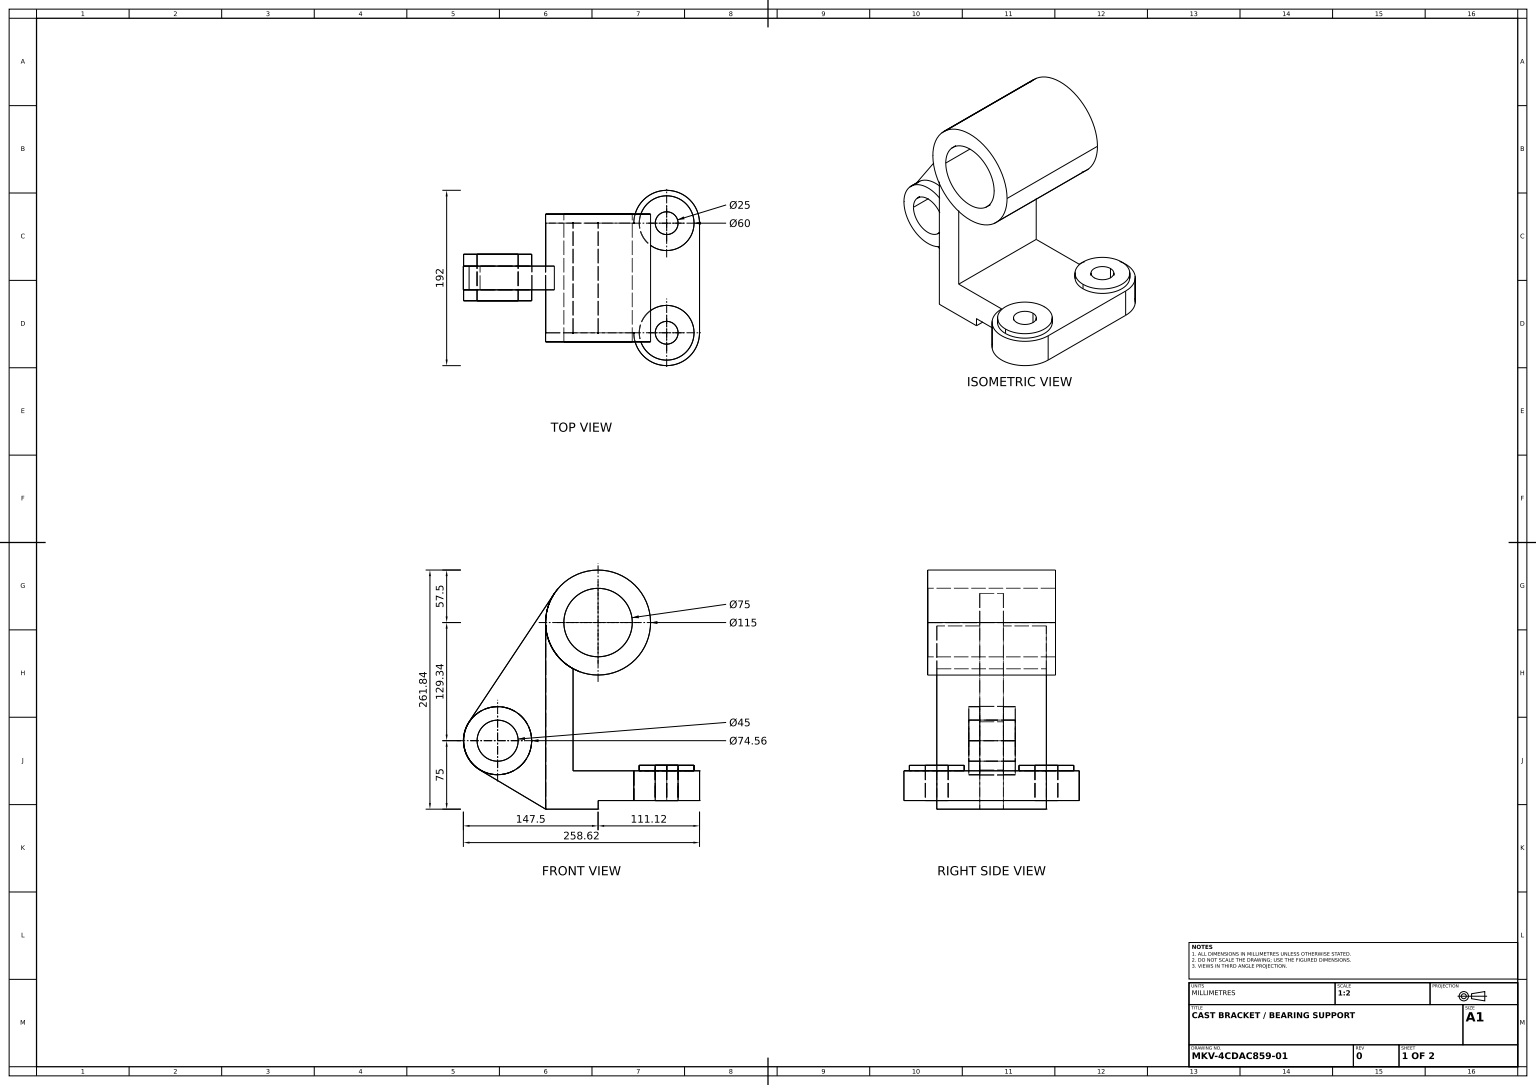
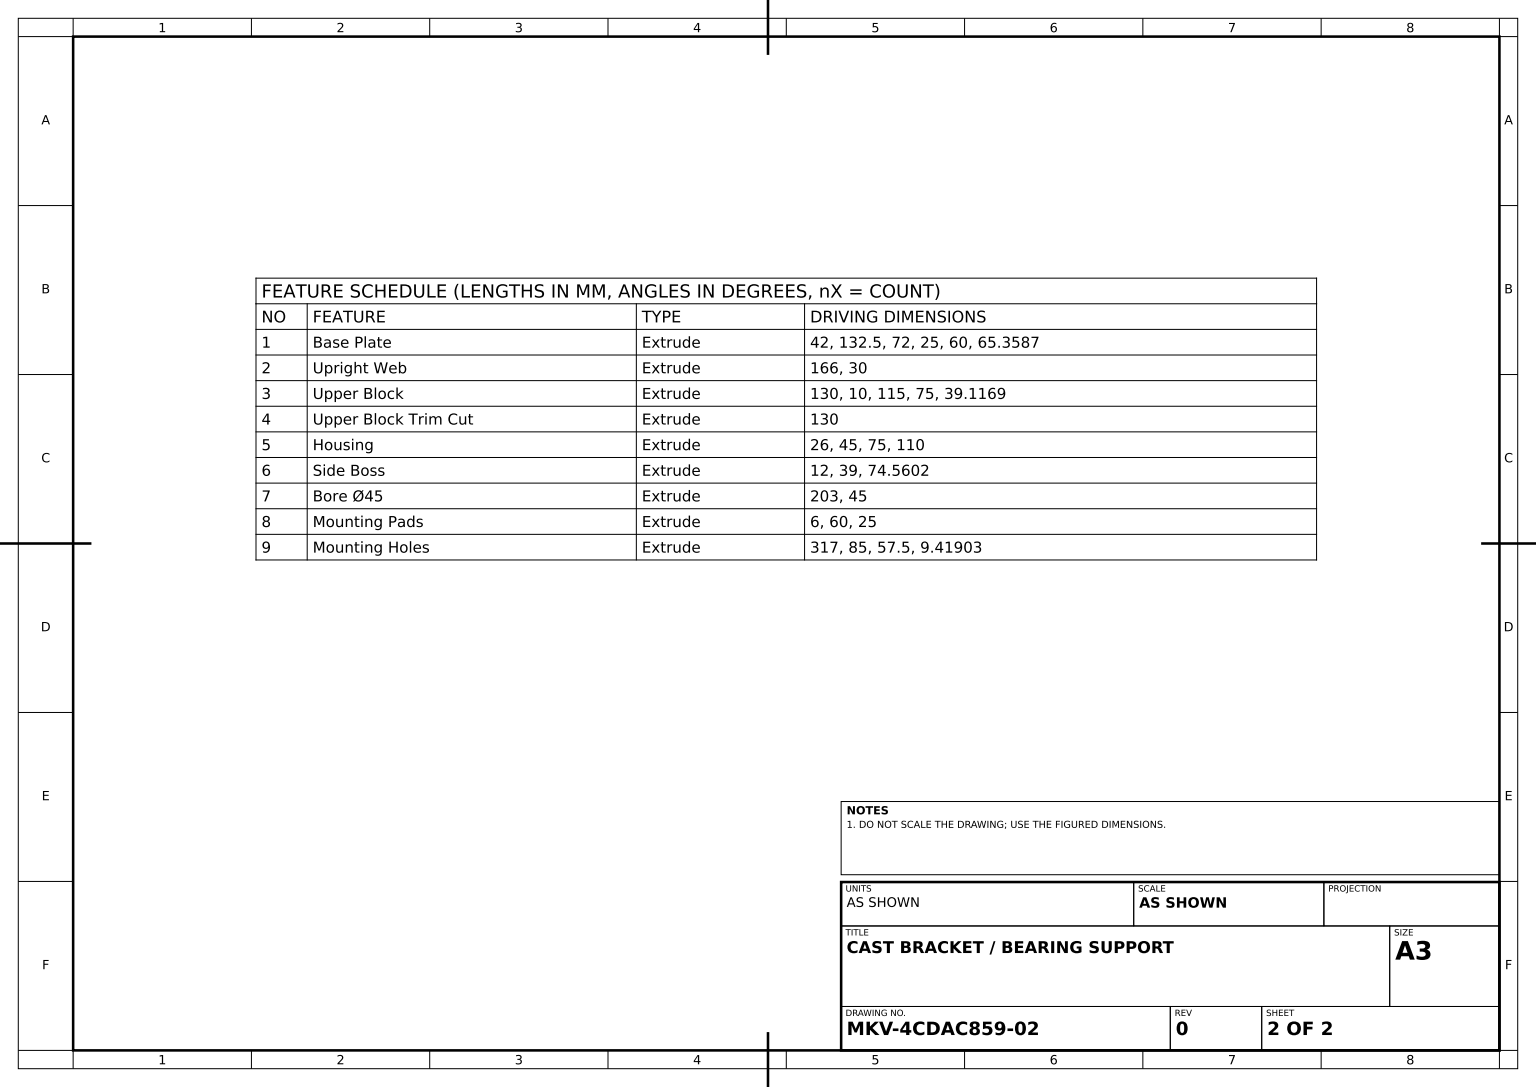
SolidWorks part; units mm, degrees
material "Plain Carbon Steel"
ref_plane "Front Plane" through (0, 0, 0) normal (0, 0, 1) x (1, 0, 0)
ref_plane "Top Plane" through (0, 0, 0) normal (0, 1, 0) x (1, 0, 0)
ref_plane "Right Plane" through (0, 0, 0) normal (1, 0, 0) x (0, 0, -1)
sketch "Base Plate Profile" plane through (0, 0, 0) normal (0, 1, 0) x (1, 0, 0)
  line L0 (0, 0) -> (20.8145, 0) construction
  line L1 (-65.3587, 60) -> (31.1413, 60)
  line L2 (-65.3587, 60) -> (-65.3587, -60)
  line L3 (-65.3587, -60) -> (31.1413, -60)
  line L5 (103.1413, 60) -> (103.1413, -60)
  arc A0 (31.1413, -60) -> (103.1413, -60) centre (67.1413, -60) ccw
  circle A1 centre (67.1413, -60) radius 12.5
  arc A2 (31.1413, 60) -> (103.1413, 60) centre (67.1413, 60) cw
  circle A3 centre (67.1413, 60) radius 12.5
  dimension "D3" = 72
  dimension "D4" = 25
  dimension "D1" = 132.5
  dimension "D2" = 65.3587
  dimension "D5" = 60
extrude "Base Plate" add sketch "Base Plate Profile" along normal blind 42
sketch "Upright Profile" plane through (0, 42, 0) normal (0, 1, 0) x (1, 0, 0)
  line L0 (-65.3587, -60) -> (31.1413, -60) construction
  line L1 (-65.3587, 60) -> (-35.3587, 60)
  line L2 (-65.3587, 60) -> (-65.3587, -60)
  line L3 (-65.3587, -60) -> (-35.3587, -60)
  line L4 (-35.3587, 60) -> (-35.3587, -60)
  dimension "D1" = 30
extrude "Upright Web" add sketch "Upright Profile" along normal blind 166
sketch "Upper Block Profile" plane through (0, 0, 60) normal (0, 0, 1) x (1, 0, 0)
  line L0 (31.1413, 42) -> (31.1413, 0) construction
  circle A0 centre (-7.9757, 204.335) radius 57.5
  circle A1 centre (-7.9757, 204.335) radius 37.5
  dimension "D1" = 115
  dimension "D2" = 75
  dimension "D3" = 39.1169
extrude "Upper Block" add sketch "Upper Block Profile" against normal blind 130 and the other way blind 10
sketch "Upper Block Trim Profile" plane through (0, 0, 60) normal (0, 0, 1) x (1, 0, 0)
  line L0 (-45.2961, 208) -> (-35.3587, 208) construction
  line L1 (-45.2961, 208) -> (-35.3587, 208)
  line L2 (-35.3587, 208) -> (-35.3587, 178.7144) construction
  line L3 (-35.3587, 208) -> (-35.3587, 178.7144)
  arc A0 (-45.2961, 208) -> (-35.3587, 178.7144) centre (-7.9757, 204.335) ccw construction
  arc A1 (-45.2961, 208) -> (-35.3587, 178.7144) centre (-7.9757, 204.335) ccw
extrude "Upper Block Trim Cut" cut sketch "Upper Block Trim Profile" against normal blind 130
sketch "Housing Profile" plane through (0, 0, 0) normal (0, 0, 1) x (1, 0, 0)
  line L0 (-137.1695, 42.7844) -> (-65.3587, 0)
  line L1 (-55.8595, 236.1688) -> (-149.2042, 95.7612)
  line L2 (-65.3587, 200.6701) -> (-65.3587, 0) construction
  line L3 (-65.3587, 200.6701) -> (-65.3587, 0)
  circle A0 centre (-117.9757, 75) radius 37.5
  circle A1 centre (-117.9757, 75) radius 22.5
  circle A2 centre (-7.9757, 204.335) radius 37.5 construction
  circle A4 centre (-7.9757, 204.335) radius 57.5 construction
  circle A5 centre (-7.9757, 204.335) radius 57.5
  dimension "D1" = 45
  dimension "D2" = 75
  dimension "D3" = 75
  dimension "D4" = 110
extrude "Housing" add sketch "Housing Profile" along normal mid plane 26 contours A5 L1 A0 L0 L3 | A0 A1
sketch "Side Boss Profile" plane through (0, 0, 13) normal (0, 0, 1) x (1, 0, 0)
  circle A0 centre (-117.9757, 75) radius 37.2801
  dimension "D1" = 74.5602
extrude "Side Boss" add sketch "Side Boss Profile" along normal blind 12 and the other way blind 39
sketch "Bore Ø45 Profile" plane through (0, 0, 25) normal (0, 0, 1) x (1, 0, 0)
  circle A0 centre (-117.9757, 75) radius 22.5
  dimension "D1" = 45
extrude "Bore Ø45" cut sketch "Bore Ø45 Profile" against normal blind 203
sketch "Mounting Pads Profile" plane through (0, 42, 0) normal (0, 1, 0) x (1, 0, 0)
  circle A0 centre (67.1413, -60) radius 30
  circle A1 centre (67.1413, 60) radius 30
  circle A2 centre (67.1413, 60) radius 12.5
  circle A3 centre (67.1413, -60) radius 12.5
  dimension "D1" = 60
  dimension "D2" = 25
extrude "Mounting Pads" add sketch "Mounting Pads Profile" along normal blind 6
sketch "Mounting Holes Profile" plane through (0, 0, 60) normal (0, 0, 1) x (1, 0, 0)
  line L0 (-65.3587, 0) -> (31.1413, 0) construction
  line L1 (-7.8587, 0) -> (103.1413, 0)
  line L2 (-7.8587, 0) -> (-7.8587, 9.419)
  line L3 (-7.8587, 9.419) -> (103.1413, 9.419)
  line L4 (103.1413, 0) -> (103.1413, 9.419)
  line L5 (103.1413, 42) -> (103.1413, 0) construction
  dimension "D1" = 57.5
  dimension "D2" = 9.419
extrude "Mounting Holes" cut sketch "Mounting Holes Profile" against normal blind 317 and the other way blind 85
